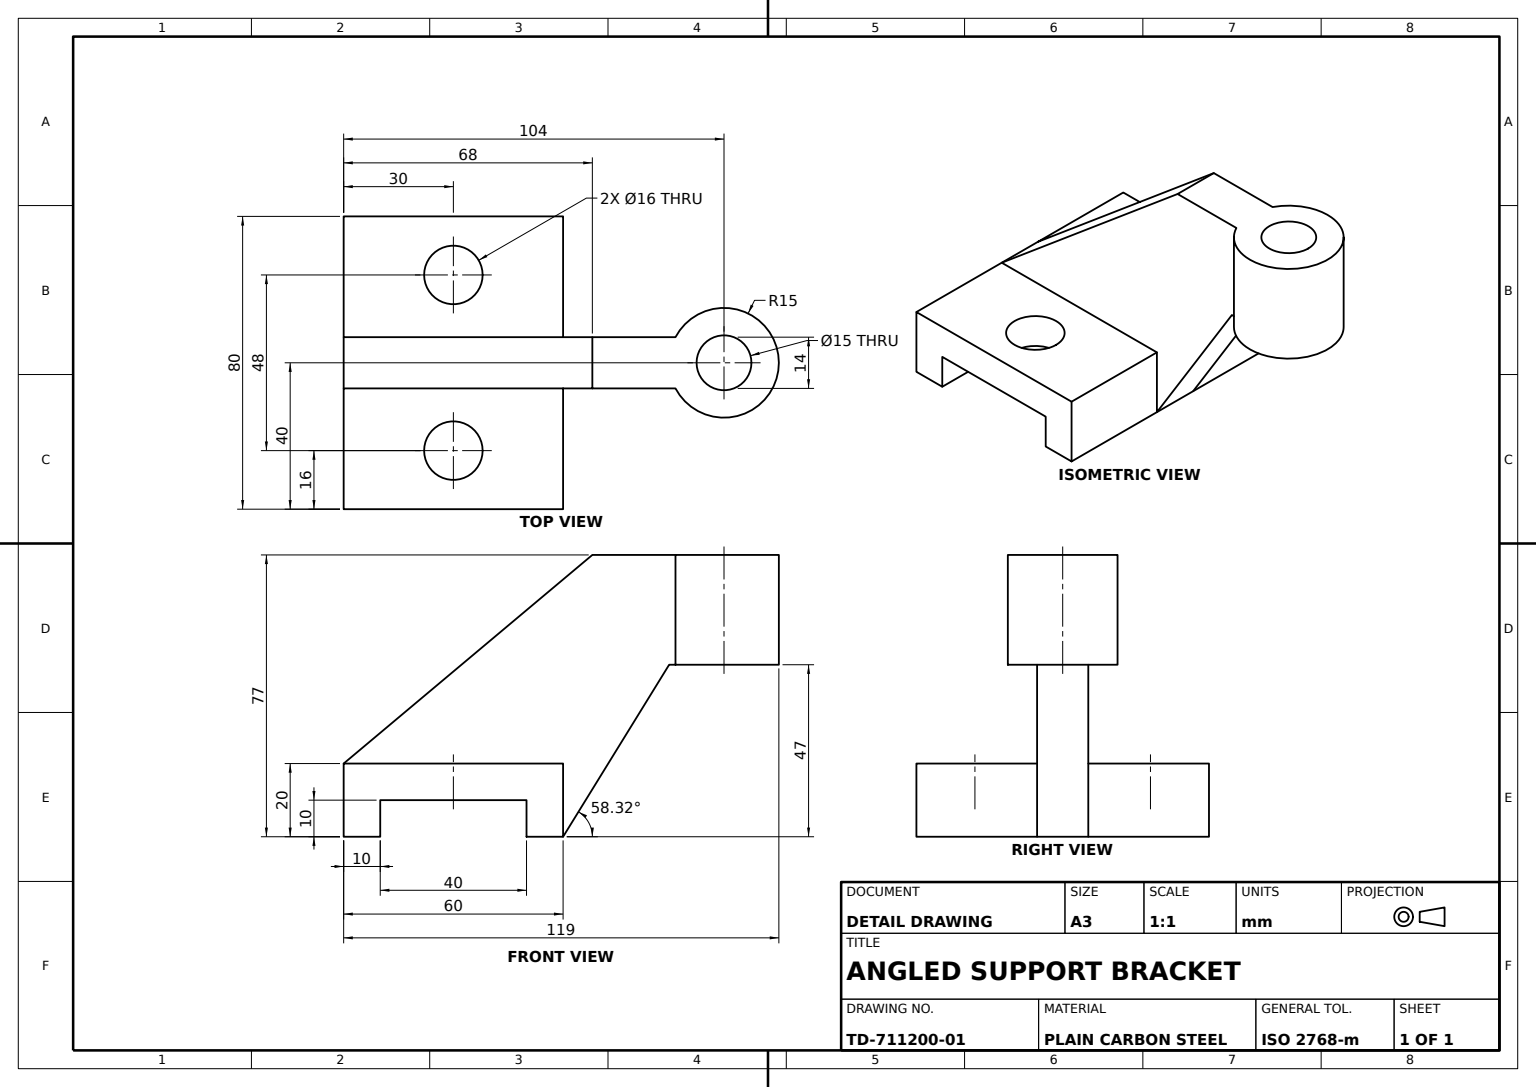
SolidWorks part; units mm, degrees
material "Plain Carbon Steel"
ref_plane "Front Plane" through (0, 0, 0) normal (0, 0, 1) x (1, 0, 0)
ref_plane "Top Plane" through (0, 0, 0) normal (0, 1, 0) x (1, 0, 0)
ref_plane "Right Plane" through (0, 0, 0) normal (1, 0, 0) x (0, 0, -1)
sketch "Base Profile Sketch" plane through (0, 0, 0) normal (0, 0, 1) x (1, 0, 0)
  line L1 (-40, 10) -> (40, 10)
  line L2 (-40, 10) -> (-40, -10)
  line L3 (-40, -10) -> (40, -10)
  line L4 (40, 10) -> (40, -10)
  line L5 (-40, 10) -> (40, -10) construction
  line L6 (-40, -10) -> (40, 10) construction
  point P0 (0, 0)
  dimension "D1" = 80
  dimension "D2" = 20
extrude "Base Block" add sketch "Base Profile Sketch" along normal mid plane 60
sketch "Round Boss Sketch" plane through (0, 10, 0) normal (0, 1, 0) x (1, 0, 0)
  line L0 (0, 74) -> (0, 0) construction
  line L1 (40, -30) -> (-40, -30) construction
  circle A0 centre (0, 74) radius 7.5
  circle A1 centre (0, 74) radius 15
  dimension "D1" = 15
  dimension "D2" = 30
  dimension "D3" = 104
extrude "Round Boss" add sketch "Round Boss Sketch" against normal blind 30 from offset 57 separate body
sketch "Inclined Arm Sketch" plane through (0, 0, 0) normal (1, 0, 0) x (0, 0, -1)
  line L0 (-30, 10) -> (38, 67)
  line L1 (38, 67) -> (59, 67)
  line L3 (59, 67) -> (59, 37) construction
  line L4 (59, 67) -> (59, 37)
  line L5 (-30, 10) -> (30, 10) construction
  line L6 (-30, 10) -> (30, 10)
  line L8 (30, -10) -> (59, 37)
  line L9 (30, -10) -> (30, 10) construction
  line L10 (30, -10) -> (30, 10)
  dimension "D1" = 68
extrude "Inclined Arm" add sketch "Inclined Arm Sketch" along normal mid plane 14
sketch "Arm Web Sketch" plane through (0, 0, -59) normal (0, 0, -1) x (-1, 0, 0)
  line L4 (-7, 37) -> (7, 37)
  line L5 (7, 37) -> (7, 67)
  line L6 (7, 67) -> (-7, 67)
  line L7 (-7, 67) -> (-7, 37)
  line L8 (-7, 37) -> (7, 37)
  line L9 (7, 37) -> (7, 67)
  line L10 (7, 67) -> (-7, 67)
  line L11 (-7, 67) -> (-7, 37)
  dimension "D1" = 0
extrude "Arm Web" add sketch "Arm Web Sketch" along normal mid plane 14
sketch "Base Slot Sketch" plane through (40, 0, 0) normal (1, 0, 0) x (0, 0, -1)
  line L0 (-30, -10) -> (30, -10) construction
  line L1 (-20, -10) -> (20, -10)
  line L2 (-20, -10) -> (-20, 0)
  line L3 (-20, 0) -> (20, 0)
  line L4 (20, -10) -> (20, 0)
  line L5 (-30, -10) -> (-30, 10) construction
  dimension "D1" = 10
  dimension "D2" = 40
  dimension "D3" = 10
extrude "Base Slot 40x10" cut sketch "Base Slot Sketch" against normal through all
sketch "Hole Cut Sketch" plane through (0, 10, 0) normal (0, 1, 0) x (1, 0, 0)
  line L0 (-7, 30) -> (-40, 30) construction
  line L1 (0, 0) -> (0, -30) construction
  line L2 (7, -30) -> (-7, -30) construction
  line L3 (-24, 0) -> (24, 0) construction
  circle A0 centre (-24, 0) radius 8
  circle A1 centre (24, 0) radius 8
  dimension "D3" = 16
  dimension "D4" = 16
  dimension "D1" = 48
  dimension "D2" = 30
  dimension "D5" = 24
extrude "Holes Ø16" cut sketch "Hole Cut Sketch" against normal through all
